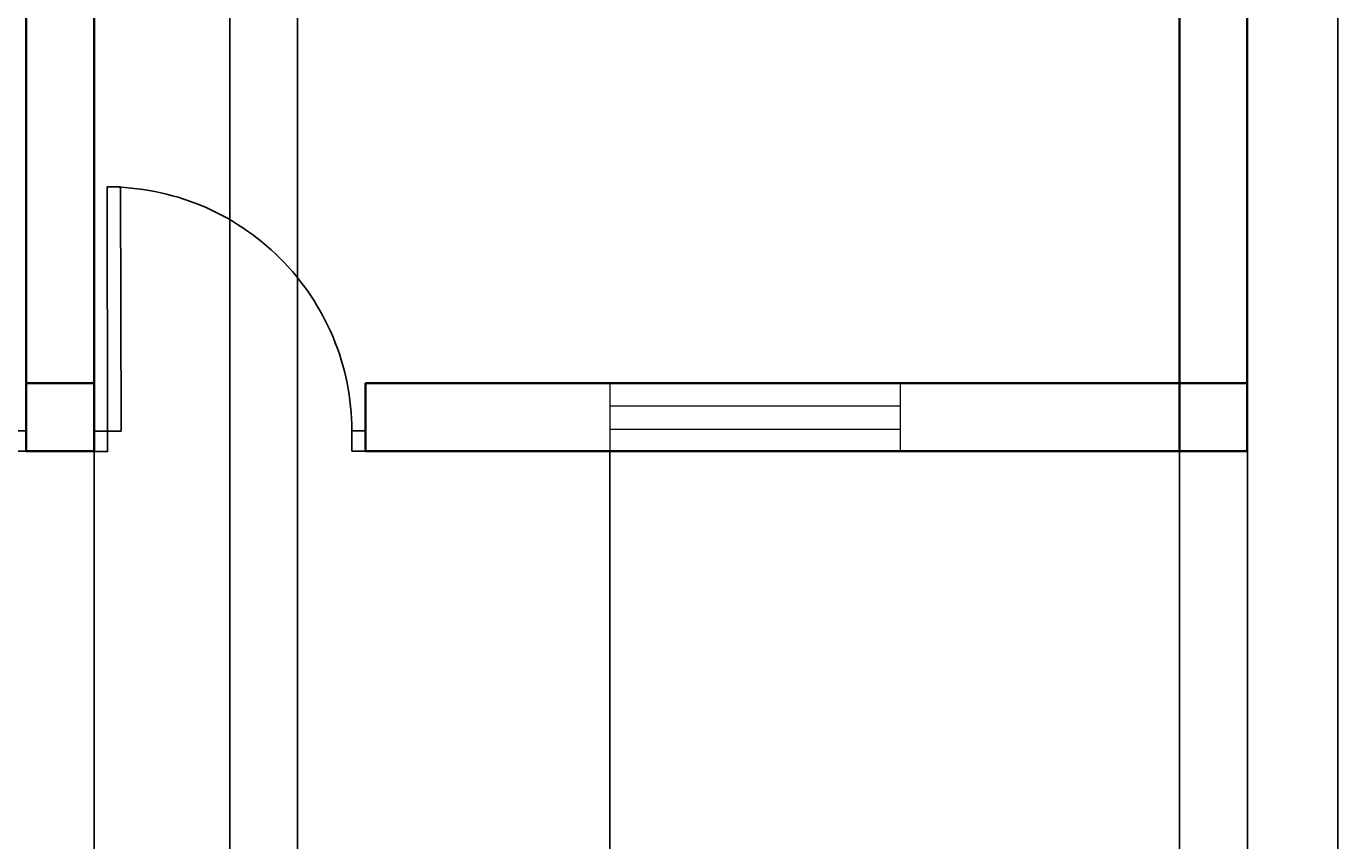
# Model space of a CAD drawing. Units: inches. Extents: x 867 to 1667, y -234 to 788.
# Tile 34 of 42: x 1221 to 1395, y 572 to 680. Entities that reach past the tile are written whole.
import ezdxf

# ---------------------------------------------------------------- set-up
doc = ezdxf.new("R2010")
doc.units = ezdxf.units.IN
doc.header["$MEASUREMENT"] = 0
for name, color, linetype, lineweight in [('A-ANNO-DIMS', 2, 'Continuous', 18), ('A-Door', 150, 'Continuous', 25), ('A-Glaz', 92, 'Continuous', 18), ('A-Wall', 7, 'Continuous', 35)]:
    doc.layers.add(name, color=color, linetype=linetype, lineweight=lineweight)
doc.layers.add('NET 01', color=8, linetype='Continuous')
doc.styles.get("Standard").update_dxf_attribs({"font": 'arial.ttf'})
doc.dimstyles.get("Standard").update_dxf_attribs({"dimtxt": 0.6875, "dimasz": 0.18, "dimexe": 0.18, "dimexo": 0.0625, "dimgap": 0.09, "dimtad": 0, "dimdec": 4, "dimzin": 0, "dimdsep": 46, "dimlunit": 4, "dimtxsty": 'Standard', "dimcen": 0.09, "dimadec": 0, "dimazin": 0, "dimtfac": 1, "dimtdec": 4, "dimtofl": 0, "dimtmove": 0, "dimatfit": 3, "dimfxl": 1, "dimtolj": 1, "dimtzin": 0, "dimarcsym": 0})

# ---------------------------------------------------------------- blocks, each defined once
blk = doc.blocks.new('A$C292B336C')
at = {"layer": 'A-Door'}
for points in [[(-0.05, 0), (-0.05, 0.9), (0, 0.9), (0, 0)], [(-0.95, 0), (-0.95, -0.075), (-0.9, -0.075), (-0.9, 0)], [(0, 0), (0, -0.075), (0.05, -0.075), (0.05, 0)]]:
    blk.add_lwpolyline(points, close=True, dxfattribs=at)
at = {"layer": 'NET 01'}
blk.add_arc((0, 0), 0.9, 90, 180, dxfattribs=at)
blk = doc.blocks.new('WIN-38_58IN')
for p, q in [((0, 9), (0, 0)), ((38.58, 0), (38.58, 9)), ((0, 6), (38.58, 6)), ((0, 2.92), (38.58, 2.92)), ((0, 0), (38.58, 0))]:
    blk.add_line(p, q)
blk = doc.blocks.new('*D23')
at = {"layer": 'A-ANNO-DIMS', "color": 0, "lineweight": -2, "transparency": 16777216}
for p, q in [((1373.89, 623.55), (1373.89, -233.54)), ((1382.89, 623.55), (1382.89, -233.54)), ((1374.07, -233.36), (1378.07, -233.36)), ((1382.71, -233.36), (1378.7, -233.36))]:
    blk.add_line(p, q, dxfattribs=at)
at = {"layer": 'A-ANNO-DIMS', "color": 0, "transparency": 16777216}
for points in [[(1374.07, -233.33), (1374.07, -233.39), (1373.89, -233.36)], [(1382.71, -233.33), (1382.71, -233.39), (1382.89, -233.36)]]:
    blk.add_solid(points, dxfattribs=at)
at = {"layer": 'Defpoints', "color": 0, "transparency": 16777216}
for p in [(1373.89, 623.62), (1382.89, 623.62), (1382.89, -233.36)]:
    blk.add_point(p, dxfattribs=at)
at = {"layer": 'A-ANNO-DIMS', "color": 0, "transparency": 16777216, "insert": (1378.39, -233.36), "char_height": 0.688, "attachment_point": 5}
blk.add_mtext('\\A1;9', dxfattribs=at)
blk = doc.blocks.new('*D30')
at = {"layer": 'A-ANNO-DIMS', "color": 0, "lineweight": -2, "transparency": 16777216}
for p, q in [((1229.89, 623.55), (1229.89, -233.54)), ((1298.3, 623.55), (1298.3, -233.54)), ((1230.07, -233.36), (1262.91, -233.36)), ((1298.12, -233.36), (1265.28, -233.36))]:
    blk.add_line(p, q, dxfattribs=at)
at = {"layer": 'A-ANNO-DIMS', "color": 0, "transparency": 16777216}
for points in [[(1230.07, -233.33), (1230.07, -233.39), (1229.89, -233.36)], [(1298.12, -233.33), (1298.12, -233.39), (1298.3, -233.36)]]:
    blk.add_solid(points, dxfattribs=at)
at = {"layer": 'Defpoints', "color": 0, "transparency": 16777216}
for p in [(1229.89, 623.62), (1298.3, 623.62), (1298.3, -233.36)]:
    blk.add_point(p, dxfattribs=at)
at = {"layer": 'A-ANNO-DIMS', "color": 0, "transparency": 16777216, "insert": (1264.09, -233.36), "char_height": 0.688, "attachment_point": 5}
blk.add_mtext('\\A1;68.41', dxfattribs=at)
blk = doc.blocks.new('*D31')
at = {"layer": 'A-ANNO-DIMS', "color": 0, "lineweight": -2, "transparency": 16777216}
for p, q in [((1070.89, 566.68), (1070.89, 787.75)), ((1071.07, 787.57), (1304.02, 787.57)), ((1538.71, 787.57), (1305.75, 787.57)), ((1538.89, 566.68), (1538.89, 787.75))]:
    blk.add_line(p, q, dxfattribs=at)
at = {"layer": 'A-ANNO-DIMS', "color": 0, "transparency": 16777216}
for points in [[(1071.07, 787.6), (1071.07, 787.54), (1070.89, 787.57)], [(1538.71, 787.6), (1538.71, 787.54), (1538.89, 787.57)]]:
    blk.add_solid(points, dxfattribs=at)
at = {"layer": 'Defpoints', "color": 0, "transparency": 16777216}
for p in [(1538.89, 787.57), (1070.89, 566.62), (1538.89, 566.62)]:
    blk.add_point(p, dxfattribs=at)
at = {"layer": 'A-ANNO-DIMS', "color": 0, "transparency": 16777216, "insert": (1304.89, 787.57), "char_height": 0.688, "attachment_point": 5}
blk.add_mtext('\\A1;468', dxfattribs=at)
blk = doc.blocks.new('*D32')
at = {"layer": 'A-ANNO-DIMS', "color": 0, "lineweight": -2, "transparency": 16777216}
for p, q in [((1079.89, 404.68), (1079.89, 787.75)), ((1080.07, 787.57), (1163.07, 787.57)), ((1247.71, 787.57), (1164.7, 787.57)), ((1247.89, 413.68), (1247.89, 787.75))]:
    blk.add_line(p, q, dxfattribs=at)
at = {"layer": 'A-ANNO-DIMS', "color": 0, "transparency": 16777216}
for points in [[(1080.07, 787.6), (1080.07, 787.54), (1079.89, 787.57)], [(1247.71, 787.6), (1247.71, 787.54), (1247.89, 787.57)]]:
    blk.add_solid(points, dxfattribs=at)
at = {"layer": 'Defpoints', "color": 0, "transparency": 16777216}
for p in [(1247.89, 787.57), (1247.89, 413.62), (1079.89, 404.62)]:
    blk.add_point(p, dxfattribs=at)
at = {"layer": 'A-ANNO-DIMS', "color": 0, "transparency": 16777216, "insert": (1163.89, 787.57), "char_height": 0.688, "attachment_point": 5}
blk.add_mtext('\\A1;168', dxfattribs=at)
blk = doc.blocks.new('*D33')
at = {"layer": 'A-ANNO-DIMS', "color": 0, "lineweight": -2, "transparency": 16777216}
for p, q in [((1256.89, 413.68), (1256.89, 787.75)), ((1257.07, 787.57), (1325.07, 787.57)), ((1394.71, 787.57), (1326.7, 787.57)), ((1394.89, 413.68), (1394.89, 787.75))]:
    blk.add_line(p, q, dxfattribs=at)
at = {"layer": 'A-ANNO-DIMS', "color": 0, "transparency": 16777216}
for points in [[(1257.07, 787.6), (1257.07, 787.54), (1256.89, 787.57)], [(1394.71, 787.6), (1394.71, 787.54), (1394.89, 787.57)]]:
    blk.add_solid(points, dxfattribs=at)
at = {"layer": 'Defpoints', "color": 0, "transparency": 16777216}
for p in [(1394.89, 787.57), (1256.89, 413.62), (1394.89, 413.62)]:
    blk.add_point(p, dxfattribs=at)
at = {"layer": 'A-ANNO-DIMS', "color": 0, "transparency": 16777216, "insert": (1325.89, 787.57), "char_height": 0.688, "attachment_point": 5}
blk.add_mtext('\\A1;138', dxfattribs=at)

msp = doc.modelspace()

# ---------------------------------------------------------------- linework, layer by layer
at = {"layer": 'A-Wall'}
for p, q in [((1220.8866, 740.617), (1220.8866, 623.617)), ((1229.8866, 740.617), (1229.8866, 623.617)), ((1373.8866, 740.617), (1373.8866, 623.617)), ((1382.8866, 740.617), (1382.8866, 623.617)), ((1229.8866, 632.617), (1220.8866, 632.617)), ((1382.8866, 632.617), (1265.8866, 632.617)), ((1265.8866, 632.617), (1265.8866, 623.617)), ((1229.8866, 623.617), (1220.8866, 623.617)), ((1382.8866, 623.617), (1265.8866, 623.617))]:
    msp.add_line(p, q, dxfattribs=at)

# ---------------------------------------------------------------- block references
at = {"layer": 'A-Door', "xscale": 36.01171521992244, "yscale": 36.01171521992244, "zscale": 36.01171521992244}
msp.add_blockref('A$C292B336C', (1219.086, 626.3179), dxfattribs=at)
at = {"layer": 'A-Door', "xscale": -36.01171521992244, "yscale": 36.01171521992244, "zscale": 36.01171521992244, "rotation": 0.1281311246168038}
msp.add_blockref('A$C292B336C', (1231.6812, 626.2434), dxfattribs=at)
at = {"layer": 'A-Glaz'}
msp.add_blockref('WIN-38_58IN', (1298.2971, 623.617), dxfattribs=at)

# ---------------------------------------------------------------- dimensions: what is measured, and where the dimension line sits
at = {"layer": 'A-ANNO-DIMS'}
for base, p1, p2, override, picture, middle in [((1538.8866, 787.567), (1070.8866, 566.617), (1538.8866, 566.617), {"dimdec": 0, "dimlfac": 1, "dimrnd": 0, "dimzin": 0, "dimdsep": 46, "dimlunit": 2}, '*D31', (1304.8866, 787.567)), ((1247.8866, 787.567), (1079.8866, 404.617), (1247.8866, 413.617), {"dimdec": 0, "dimlfac": 1, "dimrnd": 0, "dimzin": 0, "dimdsep": 46, "dimlunit": 2}, '*D32', (1163.8866, 787.567)), ((1394.8866, 787.567), (1256.8866, 413.617), (1394.8866, 413.617), {"dimdec": 0, "dimlfac": 1, "dimrnd": 0, "dimzin": 0, "dimdsep": 46, "dimlunit": 2}, '*D33', (1325.8866, 787.567)), ((1298.2966, -233.3581), (1229.8866, 623.617), (1298.2966, 623.617), {"dimdec": 2, "dimlfac": 1, "dimrnd": 0, "dimzin": 0, "dimdsep": 46, "dimlunit": 2}, '*D30', (1264.0916, -233.3581)), ((1382.8866, -233.3581), (1373.8866, 623.617), (1382.8866, 623.617), {"dimdec": 0, "dimlfac": 1, "dimrnd": 0, "dimzin": 0, "dimdsep": 46, "dimlunit": 2}, '*D23', (1378.3866, -233.3581))]:
    dim = msp.add_linear_dim(base=base, p1=p1, p2=p2, dimstyle='Standard', override=override, dxfattribs=at)
    dim.commit()
    dim.dimension.update_dxf_attribs({"geometry": picture, "text_midpoint": middle})

doc.saveas('drawing.dxf')
